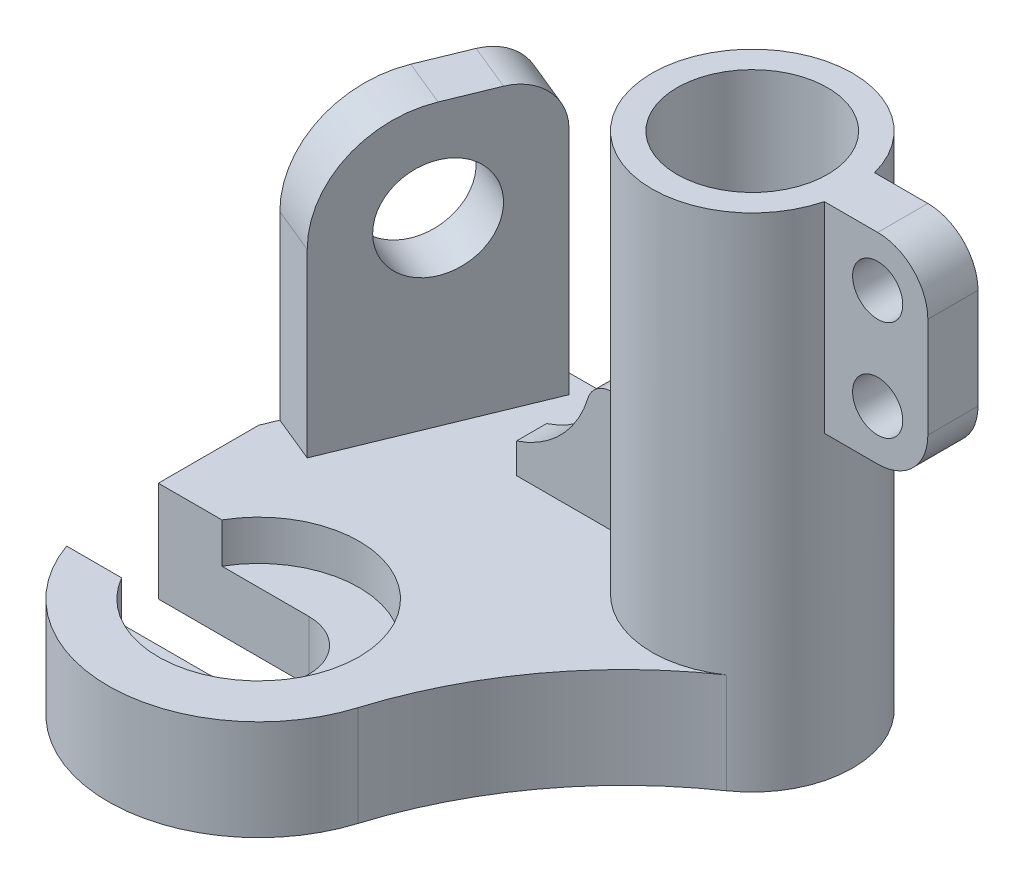
ISO-10303-21;
HEADER;
FILE_DESCRIPTION(('STEP AP214'),'2;1');
FILE_NAME('part.step','',(''),(''),'','','');
FILE_SCHEMA(('AUTOMOTIVE_DESIGN { 1 0 10303 214 1 1 1 1 }'));
ENDSEC;
DATA;
#1=APPLICATION_CONTEXT('core data for automotive mechanical design processes');
#2=APPLICATION_PROTOCOL_DEFINITION('international standard','automotive_design',2000,#1);
#3=PRODUCT_CONTEXT('',#1,'mechanical');
#4=PRODUCT('Part','Part','',(#3));
#5=PRODUCT_RELATED_PRODUCT_CATEGORY('part','',(#4));
#6=PRODUCT_DEFINITION_FORMATION('','',#4);
#7=PRODUCT_DEFINITION_CONTEXT('part definition',#1,'design');
#8=PRODUCT_DEFINITION('design','',#6,#7);
#9=PRODUCT_DEFINITION_SHAPE('','',#8);
#10=(LENGTH_UNIT() NAMED_UNIT(*) SI_UNIT(.MILLI.,.METRE.));
#11=(NAMED_UNIT(*) PLANE_ANGLE_UNIT() SI_UNIT($,.RADIAN.));
#12=(NAMED_UNIT(*) SI_UNIT($,.STERADIAN.) SOLID_ANGLE_UNIT());
#13=UNCERTAINTY_MEASURE_WITH_UNIT(LENGTH_MEASURE(1.E-05),#10,'distance_accuracy_value','');
#14=(GEOMETRIC_REPRESENTATION_CONTEXT(3) GLOBAL_UNCERTAINTY_ASSIGNED_CONTEXT((#13)) GLOBAL_UNIT_ASSIGNED_CONTEXT((#10,
#11,#12)) REPRESENTATION_CONTEXT('',''));
#15=CARTESIAN_POINT('',(0.,0.,0.));
#16=DIRECTION('',(0.,0.,1.));
#17=DIRECTION('',(1.,0.,0.));
#18=AXIS2_PLACEMENT_3D('',#15,#16,#17);
#19=CARTESIAN_POINT('',(-48.41,0.,50.));
#20=DIRECTION('',(0.,1.,0.));
#21=DIRECTION('',(0.,0.,1.));
#22=AXIS2_PLACEMENT_3D('',#19,#20,#21);
#23=CYLINDRICAL_SURFACE('',#22,10.);
#24=CARTESIAN_POINT('',(-48.41,12.,50.));
#25=DIRECTION('',(0.,1.,0.));
#26=DIRECTION('',(0.,0.,1.));
#27=AXIS2_PLACEMENT_3D('',#24,#25,#26);
#28=CIRCLE('',#27,10.);
#29=CARTESIAN_POINT('',(-48.41,12.,40.));
#30=VERTEX_POINT('',#29);
#31=CARTESIAN_POINT('',(-48.41,12.,60.));
#32=VERTEX_POINT('',#31);
#33=EDGE_CURVE('E314',#30,#32,#28,.F.);
#34=ORIENTED_EDGE('',*,*,#33,.F.);
#35=DIRECTION('',(0.,1.,0.));
#36=VECTOR('',#35,1.);
#37=CARTESIAN_POINT('',(-48.41,0.,40.));
#38=LINE('',#37,#36);
#39=CARTESIAN_POINT('',(-48.41,0.,40.));
#40=VERTEX_POINT('',#39);
#41=EDGE_CURVE('E335',#40,#30,#38,.T.);
#42=ORIENTED_EDGE('',*,*,#41,.F.);
#43=CARTESIAN_POINT('',(-48.41,0.,50.));
#44=DIRECTION('',(0.,1.,0.));
#45=DIRECTION('',(0.,0.,1.));
#46=AXIS2_PLACEMENT_3D('',#43,#44,#45);
#47=CIRCLE('',#46,10.);
#48=CARTESIAN_POINT('',(-48.41,0.,60.));
#49=VERTEX_POINT('',#48);
#50=EDGE_CURVE('E323',#49,#40,#47,.T.);
#51=ORIENTED_EDGE('',*,*,#50,.F.);
#52=DIRECTION('',(0.,1.,0.));
#53=VECTOR('',#52,1.);
#54=CARTESIAN_POINT('',(-48.41,0.,60.));
#55=LINE('',#54,#53);
#56=EDGE_CURVE('E331',#49,#32,#55,.T.);
#57=ORIENTED_EDGE('',*,*,#56,.T.);
#58=EDGE_LOOP('',(#34,#42,#51,#57));
#59=FACE_BOUND('',#58,.T.);
#60=ADVANCED_FACE('F39',(#59),#23,.F.);
#61=CARTESIAN_POINT('',(0.,100.,0.));
#62=DIRECTION('',(0.,-1.,0.));
#63=DIRECTION('',(0.,0.,-1.));
#64=AXIS2_PLACEMENT_3D('',#61,#62,#63);
#65=CYLINDRICAL_SURFACE('',#64,20.);
#66=CARTESIAN_POINT('',(0.,100.,0.));
#67=DIRECTION('',(0.,1.,0.));
#68=DIRECTION('',(0.,0.,1.));
#69=AXIS2_PLACEMENT_3D('',#66,#67,#68);
#70=CIRCLE('',#69,20.);
#71=CARTESIAN_POINT('',(19.3649167310371,100.,-5.));
#72=VERTEX_POINT('',#71);
#73=CARTESIAN_POINT('',(19.3649167310371,100.,5.));
#74=VERTEX_POINT('',#73);
#75=EDGE_CURVE('E450',#72,#74,#70,.T.);
#76=ORIENTED_EDGE('',*,*,#75,.F.);
#77=DIRECTION('',(0.,-1.,0.));
#78=VECTOR('',#77,1.);
#79=CARTESIAN_POINT('',(19.3649167310371,100.,-5.));
#80=LINE('',#79,#78);
#81=CARTESIAN_POINT('',(19.3649167310371,60.,-5.));
#82=VERTEX_POINT('',#81);
#83=EDGE_CURVE('E306',#72,#82,#80,.T.);
#84=ORIENTED_EDGE('',*,*,#83,.T.);
#85=CARTESIAN_POINT('',(0.,60.,0.));
#86=DIRECTION('',(0.,1.,0.));
#87=DIRECTION('',(0.,0.,1.));
#88=AXIS2_PLACEMENT_3D('',#85,#86,#87);
#89=CIRCLE('',#88,20.);
#90=CARTESIAN_POINT('',(19.3649167310371,60.,5.));
#91=VERTEX_POINT('',#90);
#92=EDGE_CURVE('E459',#91,#82,#89,.T.);
#93=ORIENTED_EDGE('',*,*,#92,.F.);
#94=DIRECTION('',(0.,-1.,0.));
#95=VECTOR('',#94,1.);
#96=CARTESIAN_POINT('',(19.3649167310371,100.,5.));
#97=LINE('',#96,#95);
#98=EDGE_CURVE('E303',#91,#74,#97,.F.);
#99=ORIENTED_EDGE('',*,*,#98,.T.);
#100=EDGE_LOOP('',(#76,#84,#93,#99));
#101=FACE_BOUND('',#100,.T.);
#102=CARTESIAN_POINT('',(0.,44.,0.));
#103=DIRECTION('',(0.,-1.,0.));
#104=DIRECTION('',(0.,0.,-1.));
#105=AXIS2_PLACEMENT_3D('',#102,#103,#104);
#106=CIRCLE('',#105,20.);
#107=CARTESIAN_POINT('',(-19.7737199332852,44.,3.));
#108=VERTEX_POINT('',#107);
#109=CARTESIAN_POINT('',(-19.7737199332852,44.,-3.));
#110=VERTEX_POINT('',#109);
#111=EDGE_CURVE('E11',#108,#110,#106,.T.);
#112=ORIENTED_EDGE('',*,*,#111,.F.);
#113=DIRECTION('',(0.,-1.,0.));
#114=VECTOR('',#113,1.);
#115=CARTESIAN_POINT('',(-19.7737199332852,100.,3.));
#116=LINE('',#115,#114);
#117=CARTESIAN_POINT('',(-19.7737199332852,20.,3.));
#118=VERTEX_POINT('',#117);
#119=EDGE_CURVE('E236',#108,#118,#116,.T.);
#120=ORIENTED_EDGE('',*,*,#119,.T.);
#121=CARTESIAN_POINT('',(0.,20.,0.));
#122=DIRECTION('',(0.,-1.,0.));
#123=DIRECTION('',(0.,0.,1.));
#124=AXIS2_PLACEMENT_3D('',#121,#122,#123);
#125=CIRCLE('',#124,20.);
#126=CARTESIAN_POINT('',(11.3447753734864,20.,16.4710677166095));
#127=VERTEX_POINT('',#126);
#128=EDGE_CURVE('E404',#127,#118,#125,.T.);
#129=ORIENTED_EDGE('',*,*,#128,.F.);
#130=DIRECTION('',(0.,-1.,0.));
#131=VECTOR('',#130,1.);
#132=CARTESIAN_POINT('',(11.3447753734864,20.,16.4710677166095));
#133=LINE('',#132,#131);
#134=CARTESIAN_POINT('',(11.3447753734864,0.,16.4710677166095));
#135=VERTEX_POINT('',#134);
#136=EDGE_CURVE('E419',#127,#135,#133,.T.);
#137=ORIENTED_EDGE('',*,*,#136,.T.);
#138=CARTESIAN_POINT('',(0.,0.,0.));
#139=DIRECTION('',(0.,1.,0.));
#140=DIRECTION('',(0.,0.,1.));
#141=AXIS2_PLACEMENT_3D('',#138,#139,#140);
#142=CIRCLE('',#141,20.);
#143=CARTESIAN_POINT('',(0.,0.,-20.));
#144=VERTEX_POINT('',#143);
#145=EDGE_CURVE('E447',#135,#144,#142,.T.);
#146=ORIENTED_EDGE('',*,*,#145,.T.);
#147=DIRECTION('',(0.,-1.,0.));
#148=VECTOR('',#147,1.);
#149=CARTESIAN_POINT('',(0.,20.,-20.));
#150=LINE('',#149,#148);
#151=CARTESIAN_POINT('',(0.,20.,-20.));
#152=VERTEX_POINT('',#151);
#153=EDGE_CURVE('E444',#152,#144,#150,.T.);
#154=ORIENTED_EDGE('',*,*,#153,.F.);
#155=CARTESIAN_POINT('',(-19.7737199332852,20.,-3.));
#156=VERTEX_POINT('',#155);
#157=EDGE_CURVE('E408',#156,#152,#125,.T.);
#158=ORIENTED_EDGE('',*,*,#157,.F.);
#159=DIRECTION('',(0.,-1.,0.));
#160=VECTOR('',#159,1.);
#161=CARTESIAN_POINT('',(-19.7737199332852,100.,-3.));
#162=LINE('',#161,#160);
#163=EDGE_CURVE('E53',#110,#156,#162,.T.);
#164=ORIENTED_EDGE('',*,*,#163,.F.);
#165=EDGE_LOOP('',(#112,#120,#129,#137,#146,#154,#158,#164));
#166=FACE_BOUND('',#165,.T.);
#167=ADVANCED_FACE('F489',(#101,#166),#65,.T.);
#168=CARTESIAN_POINT('',(0.,100.,0.));
#169=DIRECTION('',(0.,1.,0.));
#170=DIRECTION('',(0.,0.,1.));
#171=AXIS2_PLACEMENT_3D('',#168,#169,#170);
#172=PLANE('',#171);
#173=DIRECTION('',(1.,0.,0.));
#174=VECTOR('',#173,1.);
#175=CARTESIAN_POINT('',(18.5219863965461,100.,5.));
#176=LINE('',#175,#174);
#177=CARTESIAN_POINT('',(30.,100.,5.));
#178=VERTEX_POINT('',#177);
#179=EDGE_CURVE('E292',#74,#178,#176,.T.);
#180=ORIENTED_EDGE('',*,*,#179,.T.);
#181=DIRECTION('',(0.,0.,-1.));
#182=VECTOR('',#181,1.);
#183=CARTESIAN_POINT('',(30.,100.,0.));
#184=LINE('',#183,#182);
#185=CARTESIAN_POINT('',(30.,100.,-5.));
#186=VERTEX_POINT('',#185);
#187=EDGE_CURVE('E50',#178,#186,#184,.T.);
#188=ORIENTED_EDGE('',*,*,#187,.T.);
#189=DIRECTION('',(-1.,0.,0.));
#190=VECTOR('',#189,1.);
#191=CARTESIAN_POINT('',(18.5219863965461,100.,-5.));
#192=LINE('',#191,#190);
#193=EDGE_CURVE('E297',#186,#72,#192,.T.);
#194=ORIENTED_EDGE('',*,*,#193,.T.);
#195=ORIENTED_EDGE('',*,*,#75,.T.);
#196=EDGE_LOOP('',(#180,#188,#194,#195));
#197=FACE_BOUND('',#196,.T.);
#198=CARTESIAN_POINT('',(0.,100.,0.));
#199=DIRECTION('',(0.,1.,0.));
#200=DIRECTION('',(0.,0.,1.));
#201=AXIS2_PLACEMENT_3D('',#198,#199,#200);
#202=CIRCLE('',#201,15.);
#203=CARTESIAN_POINT('',(0.,100.,15.));
#204=VERTEX_POINT('',#203);
#205=EDGE_CURVE('E390',#204,#204,#202,.T.);
#206=ORIENTED_EDGE('',*,*,#205,.F.);
#207=EDGE_LOOP('',(#206));
#208=FACE_BOUND('',#207,.T.);
#209=ADVANCED_FACE('F479',(#197,#208),#172,.T.);
#210=CARTESIAN_POINT('',(0.,0.,0.));
#211=DIRECTION('',(0.,1.,0.));
#212=DIRECTION('',(0.,0.,1.));
#213=AXIS2_PLACEMENT_3D('',#210,#211,#212);
#214=PLANE('',#213);
#215=CARTESIAN_POINT('',(-48.41,0.,50.));
#216=DIRECTION('',(0.,1.,0.));
#217=DIRECTION('',(0.,0.,1.));
#218=AXIS2_PLACEMENT_3D('',#215,#216,#217);
#219=CIRCLE('',#218,30.);
#220=CARTESIAN_POINT('',(-76.6942712474619,0.,60.));
#221=VERTEX_POINT('',#220);
#222=CARTESIAN_POINT('',(-19.7371244907003,0.,58.8241832499221));
#223=VERTEX_POINT('',#222);
#224=EDGE_CURVE('E430',#221,#223,#219,.T.);
#225=ORIENTED_EDGE('',*,*,#224,.F.);
#226=DIRECTION('',(1.,0.,0.));
#227=VECTOR('',#226,1.);
#228=CARTESIAN_POINT('',(-48.41,0.,60.));
#229=LINE('',#228,#227);
#230=EDGE_CURVE('E328',#221,#49,#229,.T.);
#231=ORIENTED_EDGE('',*,*,#230,.T.);
#232=ORIENTED_EDGE('',*,*,#50,.T.);
#233=DIRECTION('',(-1.,0.,0.));
#234=VECTOR('',#233,1.);
#235=CARTESIAN_POINT('',(-48.41,0.,40.));
#236=LINE('',#235,#234);
#237=CARTESIAN_POINT('',(-78.41,0.,40.));
#238=VERTEX_POINT('',#237);
#239=EDGE_CURVE('E326',#40,#238,#236,.T.);
#240=ORIENTED_EDGE('',*,*,#239,.T.);
#241=DIRECTION('',(0.,0.,1.));
#242=VECTOR('',#241,1.);
#243=CARTESIAN_POINT('',(-78.41,0.,20.));
#244=LINE('',#243,#242);
#245=CARTESIAN_POINT('',(-78.41,0.,20.));
#246=VERTEX_POINT('',#245);
#247=EDGE_CURVE('E424',#246,#238,#244,.T.);
#248=ORIENTED_EDGE('',*,*,#247,.F.);
#249=DIRECTION('',(-0.379551280046691,0.,0.92517070090601));
#250=VECTOR('',#249,1.);
#251=CARTESIAN_POINT('',(-62.,0.,-20.));
#252=LINE('',#251,#250);
#253=CARTESIAN_POINT('',(-62.,0.,-20.));
#254=VERTEX_POINT('',#253);
#255=EDGE_CURVE('E425',#254,#246,#252,.T.);
#256=ORIENTED_EDGE('',*,*,#255,.F.);
#257=DIRECTION('',(-1.,0.,0.));
#258=VECTOR('',#257,1.);
#259=CARTESIAN_POINT('',(0.,0.,-20.));
#260=LINE('',#259,#258);
#261=EDGE_CURVE('E401',#144,#254,#260,.T.);
#262=ORIENTED_EDGE('',*,*,#261,.F.);
#263=ORIENTED_EDGE('',*,*,#145,.F.);
#264=CARTESIAN_POINT('',(56.723876867432,0.,82.3553385830477));
#265=DIRECTION('',(0.,-1.,0.));
#266=DIRECTION('',(0.,0.,-1.));
#267=AXIS2_PLACEMENT_3D('',#264,#265,#266);
#268=CIRCLE('',#267,80.);
#269=EDGE_CURVE('E427',#223,#135,#268,.T.);
#270=ORIENTED_EDGE('',*,*,#269,.F.);
#271=EDGE_LOOP('',(#225,#231,#232,#240,#248,#256,#262,#263,#270));
#272=FACE_BOUND('',#271,.T.);
#273=ADVANCED_FACE('F586',(#272),#214,.F.);
#274=CARTESIAN_POINT('',(0.,20.,-20.));
#275=DIRECTION('',(0.,0.,1.));
#276=DIRECTION('',(1.,0.,0.));
#277=AXIS2_PLACEMENT_3D('',#274,#275,#276);
#278=PLANE('',#277);
#279=ORIENTED_EDGE('',*,*,#261,.T.);
#280=DIRECTION('',(0.,-1.,0.));
#281=VECTOR('',#280,1.);
#282=CARTESIAN_POINT('',(-62.,20.,-20.));
#283=LINE('',#282,#281);
#284=CARTESIAN_POINT('',(-62.,20.,-20.));
#285=VERTEX_POINT('',#284);
#286=EDGE_CURVE('E439',#285,#254,#283,.T.);
#287=ORIENTED_EDGE('',*,*,#286,.F.);
#288=DIRECTION('',(-1.,0.,0.));
#289=VECTOR('',#288,1.);
#290=CARTESIAN_POINT('',(0.,20.,-20.));
#291=LINE('',#290,#289);
#292=EDGE_CURVE('E410',#152,#285,#291,.T.);
#293=ORIENTED_EDGE('',*,*,#292,.F.);
#294=ORIENTED_EDGE('',*,*,#153,.T.);
#295=EDGE_LOOP('',(#279,#287,#293,#294));
#296=FACE_BOUND('',#295,.T.);
#297=ADVANCED_FACE('F585',(#296),#278,.F.);
#298=CARTESIAN_POINT('',(-62.,20.,-20.));
#299=DIRECTION('',(0.925170700906011,0.,0.379551280046691));
#300=DIRECTION('',(0.379551280046691,0.,-0.925170700906011));
#301=AXIS2_PLACEMENT_3D('',#298,#299,#300);
#302=PLANE('',#301);
#303=ORIENTED_EDGE('',*,*,#255,.T.);
#304=DIRECTION('',(0.,-1.,0.));
#305=VECTOR('',#304,1.);
#306=CARTESIAN_POINT('',(-78.41,20.,20.));
#307=LINE('',#306,#305);
#308=CARTESIAN_POINT('',(-78.41,20.,20.));
#309=VERTEX_POINT('',#308);
#310=EDGE_CURVE('E440',#309,#246,#307,.T.);
#311=ORIENTED_EDGE('',*,*,#310,.F.);
#312=DIRECTION('',(-0.379551280046691,0.,0.92517070090601));
#313=VECTOR('',#312,1.);
#314=CARTESIAN_POINT('',(-62.,20.,-20.));
#315=LINE('',#314,#313);
#316=CARTESIAN_POINT('',(-77.1820512018676,20.,17.0068280362404));
#317=VERTEX_POINT('',#316);
#318=EDGE_CURVE('E406',#317,#309,#315,.T.);
#319=ORIENTED_EDGE('',*,*,#318,.F.);
#320=DIRECTION('',(0.,1.,0.));
#321=VECTOR('',#320,1.);
#322=CARTESIAN_POINT('',(-77.1820512018676,56.,17.0068280362404));
#323=LINE('',#322,#321);
#324=CARTESIAN_POINT('',(-77.1820512018676,56.,17.0068280362404));
#325=VERTEX_POINT('',#324);
#326=EDGE_CURVE('E349',#317,#325,#323,.T.);
#327=ORIENTED_EDGE('',*,*,#326,.T.);
#328=CARTESIAN_POINT('',(-69.5910256009338,56.,-1.49658598187978));
#329=DIRECTION('',(-0.925170700906011,0.,-0.379551280046691));
#330=DIRECTION('',(0.379551280046691,0.,-0.925170700906011));
#331=AXIS2_PLACEMENT_3D('',#328,#329,#330);
#332=CIRCLE('',#331,20.);
#333=CARTESIAN_POINT('',(-69.5910256009338,76.,-1.49658598187978));
#334=VERTEX_POINT('',#333);
#335=EDGE_CURVE('E373',#325,#334,#332,.T.);
#336=ORIENTED_EDGE('',*,*,#335,.T.);
#337=DIRECTION('',(0.379551280046691,0.,-0.92517070090601));
#338=VECTOR('',#337,1.);
#339=CARTESIAN_POINT('',(-65.7955128004669,76.,-10.7482929909398));
#340=LINE('',#339,#338);
#341=CARTESIAN_POINT('',(-65.7955128004669,76.,-10.7482929909398));
#342=VERTEX_POINT('',#341);
#343=EDGE_CURVE('E376',#334,#342,#340,.T.);
#344=ORIENTED_EDGE('',*,*,#343,.T.);
#345=CARTESIAN_POINT('',(-65.7955128004669,66.,-10.7482929909399));
#346=DIRECTION('',(-0.925170700906011,0.,-0.379551280046691));
#347=DIRECTION('',(0.379551280046691,0.,-0.925170700906011));
#348=AXIS2_PLACEMENT_3D('',#345,#346,#347);
#349=CIRCLE('',#348,10.);
#350=CARTESIAN_POINT('',(-62.,65.9999999999999,-20.));
#351=VERTEX_POINT('',#350);
#352=EDGE_CURVE('E377',#342,#351,#349,.T.);
#353=ORIENTED_EDGE('',*,*,#352,.T.);
#354=DIRECTION('',(0.,-1.,0.));
#355=VECTOR('',#354,1.);
#356=CARTESIAN_POINT('',(-62.,20.,-20.));
#357=LINE('',#356,#355);
#358=EDGE_CURVE('E351',#351,#285,#357,.T.);
#359=ORIENTED_EDGE('',*,*,#358,.T.);
#360=ORIENTED_EDGE('',*,*,#286,.T.);
#361=EDGE_LOOP('',(#303,#311,#319,#327,#336,#344,#353,#359,#360));
#362=FACE_BOUND('',#361,.T.);
#363=CARTESIAN_POINT('',(-69.5910256009338,56.,-1.49658598187978));
#364=DIRECTION('',(-0.925170700906011,0.,-0.379551280046691));
#365=DIRECTION('',(-0.379551280046691,0.,0.925170700906011));
#366=AXIS2_PLACEMENT_3D('',#363,#364,#365);
#367=CIRCLE('',#366,10.);
#368=CARTESIAN_POINT('',(-73.3865384014007,56.,7.75512102718032));
#369=VERTEX_POINT('',#368);
#370=EDGE_CURVE('E342',#369,#369,#367,.T.);
#371=ORIENTED_EDGE('',*,*,#370,.F.);
#372=EDGE_LOOP('',(#371));
#373=FACE_BOUND('',#372,.T.);
#374=ADVANCED_FACE('F577',(#362,#373),#302,.F.);
#375=CARTESIAN_POINT('',(-78.41,20.,20.));
#376=DIRECTION('',(1.,0.,0.));
#377=DIRECTION('',(0.,0.,-1.));
#378=AXIS2_PLACEMENT_3D('',#375,#376,#377);
#379=PLANE('',#378);
#380=ORIENTED_EDGE('',*,*,#247,.T.);
#381=DIRECTION('',(0.,1.,0.));
#382=VECTOR('',#381,1.);
#383=CARTESIAN_POINT('',(-78.41,0.,40.));
#384=LINE('',#383,#382);
#385=CARTESIAN_POINT('',(-78.41,20.,40.));
#386=VERTEX_POINT('',#385);
#387=EDGE_CURVE('E338',#238,#386,#384,.T.);
#388=ORIENTED_EDGE('',*,*,#387,.T.);
#389=DIRECTION('',(0.,0.,1.));
#390=VECTOR('',#389,1.);
#391=CARTESIAN_POINT('',(-78.41,20.,20.));
#392=LINE('',#391,#390);
#393=EDGE_CURVE('E411',#309,#386,#392,.T.);
#394=ORIENTED_EDGE('',*,*,#393,.F.);
#395=ORIENTED_EDGE('',*,*,#310,.T.);
#396=EDGE_LOOP('',(#380,#388,#394,#395));
#397=FACE_BOUND('',#396,.T.);
#398=ADVANCED_FACE('F579',(#397),#379,.F.);
#399=CARTESIAN_POINT('',(-48.41,20.,50.));
#400=DIRECTION('',(0.,-1.,0.));
#401=DIRECTION('',(0.,0.,-1.));
#402=AXIS2_PLACEMENT_3D('',#399,#400,#401);
#403=CYLINDRICAL_SURFACE('',#402,30.);
#404=CARTESIAN_POINT('',(-48.41,20.,50.));
#405=DIRECTION('',(0.,1.,0.));
#406=DIRECTION('',(0.,0.,1.));
#407=AXIS2_PLACEMENT_3D('',#404,#405,#406);
#408=CIRCLE('',#407,30.);
#409=CARTESIAN_POINT('',(-76.6942712474619,20.,60.));
#410=VERTEX_POINT('',#409);
#411=CARTESIAN_POINT('',(-19.7371244907003,20.,58.8241832499221));
#412=VERTEX_POINT('',#411);
#413=EDGE_CURVE('E412',#410,#412,#408,.T.);
#414=ORIENTED_EDGE('',*,*,#413,.F.);
#415=DIRECTION('',(0.,-1.,0.));
#416=VECTOR('',#415,1.);
#417=CARTESIAN_POINT('',(-76.6942712474619,20.,60.));
#418=LINE('',#417,#416);
#419=EDGE_CURVE('E340',#410,#221,#418,.T.);
#420=ORIENTED_EDGE('',*,*,#419,.T.);
#421=ORIENTED_EDGE('',*,*,#224,.T.);
#422=DIRECTION('',(0.,-1.,0.));
#423=VECTOR('',#422,1.);
#424=CARTESIAN_POINT('',(-19.7371244907003,20.,58.8241832499221));
#425=LINE('',#424,#423);
#426=EDGE_CURVE('E432',#412,#223,#425,.T.);
#427=ORIENTED_EDGE('',*,*,#426,.F.);
#428=EDGE_LOOP('',(#414,#420,#421,#427));
#429=FACE_BOUND('',#428,.T.);
#430=ADVANCED_FACE('F573',(#429),#403,.T.);
#431=CARTESIAN_POINT('',(56.723876867432,20.,82.3553385830477));
#432=DIRECTION('',(0.,-1.,0.));
#433=DIRECTION('',(0.,0.,-1.));
#434=AXIS2_PLACEMENT_3D('',#431,#432,#433);
#435=CYLINDRICAL_SURFACE('',#434,80.);
#436=ORIENTED_EDGE('',*,*,#269,.T.);
#437=ORIENTED_EDGE('',*,*,#136,.F.);
#438=CARTESIAN_POINT('',(56.723876867432,20.,82.3553385830477));
#439=DIRECTION('',(0.,-1.,0.));
#440=DIRECTION('',(0.,0.,-1.));
#441=AXIS2_PLACEMENT_3D('',#438,#439,#440);
#442=CIRCLE('',#441,80.);
#443=EDGE_CURVE('E417',#412,#127,#442,.T.);
#444=ORIENTED_EDGE('',*,*,#443,.F.);
#445=ORIENTED_EDGE('',*,*,#426,.T.);
#446=EDGE_LOOP('',(#436,#437,#444,#445));
#447=FACE_BOUND('',#446,.T.);
#448=ADVANCED_FACE('F569',(#447),#435,.F.);
#449=CARTESIAN_POINT('',(0.,20.,0.));
#450=DIRECTION('',(0.,1.,0.));
#451=DIRECTION('',(0.,0.,1.));
#452=AXIS2_PLACEMENT_3D('',#449,#450,#451);
#453=PLANE('',#452);
#454=DIRECTION('',(1.,0.,0.));
#455=VECTOR('',#454,1.);
#456=CARTESIAN_POINT('',(-44.,20.,3.));
#457=LINE('',#456,#455);
#458=CARTESIAN_POINT('',(-44.,20.,3.));
#459=VERTEX_POINT('',#458);
#460=EDGE_CURVE('E242',#459,#118,#457,.T.);
#461=ORIENTED_EDGE('',*,*,#460,.F.);
#462=DIRECTION('',(0.,0.,-1.));
#463=VECTOR('',#462,1.);
#464=CARTESIAN_POINT('',(-44.,20.,3.));
#465=LINE('',#464,#463);
#466=CARTESIAN_POINT('',(-44.,20.,-3.));
#467=VERTEX_POINT('',#466);
#468=EDGE_CURVE('E261',#459,#467,#465,.T.);
#469=ORIENTED_EDGE('',*,*,#468,.T.);
#470=DIRECTION('',(1.,0.,0.));
#471=VECTOR('',#470,1.);
#472=CARTESIAN_POINT('',(-44.,20.,-3.));
#473=LINE('',#472,#471);
#474=EDGE_CURVE('E265',#467,#156,#473,.T.);
#475=ORIENTED_EDGE('',*,*,#474,.T.);
#476=ORIENTED_EDGE('',*,*,#157,.T.);
#477=ORIENTED_EDGE('',*,*,#292,.T.);
#478=DIRECTION('',(-0.925170700906011,0.,-0.379551280046691));
#479=VECTOR('',#478,1.);
#480=CARTESIAN_POINT('',(-52.7482929909399,20.,-16.2044871995331));
#481=LINE('',#480,#479);
#482=CARTESIAN_POINT('',(-52.7482929909399,20.,-16.2044871995331));
#483=VERTEX_POINT('',#482);
#484=EDGE_CURVE('E383',#483,#285,#481,.T.);
#485=ORIENTED_EDGE('',*,*,#484,.F.);
#486=DIRECTION('',(-0.379551280046691,0.,0.92517070090601));
#487=VECTOR('',#486,1.);
#488=CARTESIAN_POINT('',(-67.9303441928075,20.,20.8023408367073));
#489=LINE('',#488,#487);
#490=CARTESIAN_POINT('',(-67.9303441928075,20.,20.8023408367073));
#491=VERTEX_POINT('',#490);
#492=EDGE_CURVE('E355',#483,#491,#489,.T.);
#493=ORIENTED_EDGE('',*,*,#492,.T.);
#494=DIRECTION('',(-0.925170700906011,0.,-0.379551280046691));
#495=VECTOR('',#494,1.);
#496=CARTESIAN_POINT('',(-67.9303441928075,20.,20.8023408367073));
#497=LINE('',#496,#495);
#498=EDGE_CURVE('E367',#491,#317,#497,.T.);
#499=ORIENTED_EDGE('',*,*,#498,.T.);
#500=ORIENTED_EDGE('',*,*,#318,.T.);
#501=ORIENTED_EDGE('',*,*,#393,.T.);
#502=DIRECTION('',(-1.,0.,0.));
#503=VECTOR('',#502,1.);
#504=CARTESIAN_POINT('',(-48.41,20.,40.));
#505=LINE('',#504,#503);
#506=CARTESIAN_POINT('',(-65.7305080756888,20.,40.));
#507=VERTEX_POINT('',#506);
#508=EDGE_CURVE('E325',#507,#386,#505,.T.);
#509=ORIENTED_EDGE('',*,*,#508,.F.);
#510=CARTESIAN_POINT('',(-48.41,20.,50.));
#511=DIRECTION('',(0.,1.,0.));
#512=DIRECTION('',(0.,0.,1.));
#513=AXIS2_PLACEMENT_3D('',#510,#511,#512);
#514=CIRCLE('',#513,20.);
#515=CARTESIAN_POINT('',(-65.7305080756888,20.,60.));
#516=VERTEX_POINT('',#515);
#517=EDGE_CURVE('E313',#516,#507,#514,.T.);
#518=ORIENTED_EDGE('',*,*,#517,.F.);
#519=DIRECTION('',(1.,0.,0.));
#520=VECTOR('',#519,1.);
#521=CARTESIAN_POINT('',(0.,20.,60.));
#522=LINE('',#521,#520);
#523=EDGE_CURVE('E446',#410,#516,#522,.T.);
#524=ORIENTED_EDGE('',*,*,#523,.F.);
#525=ORIENTED_EDGE('',*,*,#413,.T.);
#526=ORIENTED_EDGE('',*,*,#443,.T.);
#527=ORIENTED_EDGE('',*,*,#128,.T.);
#528=EDGE_LOOP('',(#461,#469,#475,#476,#477,#485,#493,#499,#500,#501,#509,#518,#524,#525,#526,#527));
#529=FACE_BOUND('',#528,.T.);
#530=ADVANCED_FACE('F562',(#529),#453,.T.);
#531=CARTESIAN_POINT('',(0.,58.,0.));
#532=DIRECTION('',(0.,1.,0.));
#533=DIRECTION('',(0.,0.,1.));
#534=AXIS2_PLACEMENT_3D('',#531,#532,#533);
#535=CONICAL_SURFACE('',#534,15.,1.02974425867665);
#536=CARTESIAN_POINT('',(0.,48.9870907145866,0.));
#537=VERTEX_POINT('',#536);
#538=VERTEX_LOOP('',#537);
#539=FACE_BOUND('',#538,.T.);
#540=CARTESIAN_POINT('',(0.,58.,0.));
#541=DIRECTION('',(0.,1.,0.));
#542=DIRECTION('',(0.,0.,1.));
#543=AXIS2_PLACEMENT_3D('',#540,#541,#542);
#544=CIRCLE('',#543,15.);
#545=CARTESIAN_POINT('',(0.,58.,15.));
#546=VERTEX_POINT('',#545);
#547=EDGE_CURVE('E397',#546,#546,#544,.T.);
#548=ORIENTED_EDGE('',*,*,#547,.T.);
#549=EDGE_LOOP('',(#548));
#550=FACE_BOUND('',#549,.T.);
#551=ADVANCED_FACE('F564',(#539,#550),#535,.F.);
#552=CARTESIAN_POINT('',(0.,100.,0.));
#553=DIRECTION('',(0.,1.,0.));
#554=DIRECTION('',(0.,0.,1.));
#555=AXIS2_PLACEMENT_3D('',#552,#553,#554);
#556=CYLINDRICAL_SURFACE('',#555,15.);
#557=ORIENTED_EDGE('',*,*,#547,.F.);
#558=EDGE_LOOP('',(#557));
#559=FACE_BOUND('',#558,.T.);
#560=ORIENTED_EDGE('',*,*,#205,.T.);
#561=EDGE_LOOP('',(#560));
#562=FACE_BOUND('',#561,.T.);
#563=ADVANCED_FACE('F543',(#559,#562),#556,.F.);
#564=CARTESIAN_POINT('',(-52.7482929909399,20.,-16.2044871995331));
#565=DIRECTION('',(0.379551280046691,0.,-0.925170700906011));
#566=DIRECTION('',(-0.925170700906011,0.,-0.379551280046691));
#567=AXIS2_PLACEMENT_3D('',#564,#565,#566);
#568=PLANE('',#567);
#569=ORIENTED_EDGE('',*,*,#358,.F.);
#570=DIRECTION('',(-0.925170700906011,0.,-0.379551280046691));
#571=VECTOR('',#570,1.);
#572=CARTESIAN_POINT('',(-52.7482929909399,65.9999999999999,-16.2044871995331));
#573=LINE('',#572,#571);
#574=CARTESIAN_POINT('',(-52.7482929909399,65.9999999999999,-16.2044871995331));
#575=VERTEX_POINT('',#574);
#576=EDGE_CURVE('E389',#575,#351,#573,.T.);
#577=ORIENTED_EDGE('',*,*,#576,.F.);
#578=DIRECTION('',(0.,-1.,0.));
#579=VECTOR('',#578,1.);
#580=CARTESIAN_POINT('',(-52.7482929909399,20.,-16.2044871995331));
#581=LINE('',#580,#579);
#582=EDGE_CURVE('E370',#575,#483,#581,.T.);
#583=ORIENTED_EDGE('',*,*,#582,.T.);
#584=ORIENTED_EDGE('',*,*,#484,.T.);
#585=EDGE_LOOP('',(#569,#577,#583,#584));
#586=FACE_BOUND('',#585,.T.);
#587=ADVANCED_FACE('F537',(#586),#568,.T.);
#588=CARTESIAN_POINT('',(-56.5438057914068,66.,-6.95278019047298));
#589=DIRECTION('',(-0.925170700906011,0.,-0.379551280046691));
#590=DIRECTION('',(-0.379551280046691,0.,0.925170700906011));
#591=AXIS2_PLACEMENT_3D('',#588,#589,#590);
#592=CYLINDRICAL_SURFACE('',#591,10.);
#593=ORIENTED_EDGE('',*,*,#352,.F.);
#594=DIRECTION('',(-0.925170700906011,0.,-0.379551280046691));
#595=VECTOR('',#594,1.);
#596=CARTESIAN_POINT('',(-56.5438057914068,76.,-6.95278019047292));
#597=LINE('',#596,#595);
#598=CARTESIAN_POINT('',(-56.5438057914068,76.,-6.95278019047292));
#599=VERTEX_POINT('',#598);
#600=EDGE_CURVE('E388',#599,#342,#597,.T.);
#601=ORIENTED_EDGE('',*,*,#600,.F.);
#602=CARTESIAN_POINT('',(-56.5438057914068,66.,-6.95278019047298));
#603=DIRECTION('',(-0.925170700906011,0.,-0.379551280046691));
#604=DIRECTION('',(0.379551280046691,0.,-0.925170700906011));
#605=AXIS2_PLACEMENT_3D('',#602,#603,#604);
#606=CIRCLE('',#605,10.);
#607=EDGE_CURVE('E365',#599,#575,#606,.T.);
#608=ORIENTED_EDGE('',*,*,#607,.T.);
#609=ORIENTED_EDGE('',*,*,#576,.T.);
#610=EDGE_LOOP('',(#593,#601,#608,#609));
#611=FACE_BOUND('',#610,.T.);
#612=ADVANCED_FACE('F545',(#611),#592,.T.);
#613=CARTESIAN_POINT('',(-56.5438057914068,76.,-6.95278019047292));
#614=DIRECTION('',(0.,1.,0.));
#615=DIRECTION('',(0.,0.,1.));
#616=AXIS2_PLACEMENT_3D('',#613,#614,#615);
#617=PLANE('',#616);
#618=ORIENTED_EDGE('',*,*,#343,.F.);
#619=DIRECTION('',(-0.925170700906011,0.,-0.379551280046691));
#620=VECTOR('',#619,1.);
#621=CARTESIAN_POINT('',(-60.3393185918737,76.,2.29892681858712));
#622=LINE('',#621,#620);
#623=CARTESIAN_POINT('',(-60.3393185918737,76.,2.29892681858712));
#624=VERTEX_POINT('',#623);
#625=EDGE_CURVE('E395',#624,#334,#622,.T.);
#626=ORIENTED_EDGE('',*,*,#625,.F.);
#627=DIRECTION('',(0.379551280046691,0.,-0.92517070090601));
#628=VECTOR('',#627,1.);
#629=CARTESIAN_POINT('',(-56.5438057914068,76.,-6.95278019047292));
#630=LINE('',#629,#628);
#631=EDGE_CURVE('E363',#624,#599,#630,.T.);
#632=ORIENTED_EDGE('',*,*,#631,.T.);
#633=ORIENTED_EDGE('',*,*,#600,.T.);
#634=EDGE_LOOP('',(#618,#626,#632,#633));
#635=FACE_BOUND('',#634,.T.);
#636=ADVANCED_FACE('F550',(#635),#617,.T.);
#637=CARTESIAN_POINT('',(-60.3393185918737,56.,2.29892681858712));
#638=DIRECTION('',(-0.925170700906011,0.,-0.379551280046691));
#639=DIRECTION('',(-0.379551280046691,0.,0.925170700906011));
#640=AXIS2_PLACEMENT_3D('',#637,#638,#639);
#641=CYLINDRICAL_SURFACE('',#640,20.);
#642=ORIENTED_EDGE('',*,*,#335,.F.);
#643=DIRECTION('',(-0.925170700906011,0.,-0.379551280046691));
#644=VECTOR('',#643,1.);
#645=CARTESIAN_POINT('',(-67.9303441928075,56.,20.8023408367073));
#646=LINE('',#645,#644);
#647=CARTESIAN_POINT('',(-67.9303441928075,56.,20.8023408367073));
#648=VERTEX_POINT('',#647);
#649=EDGE_CURVE('E394',#648,#325,#646,.T.);
#650=ORIENTED_EDGE('',*,*,#649,.F.);
#651=CARTESIAN_POINT('',(-60.3393185918737,56.,2.29892681858712));
#652=DIRECTION('',(-0.925170700906011,0.,-0.379551280046691));
#653=DIRECTION('',(0.379551280046691,0.,-0.925170700906011));
#654=AXIS2_PLACEMENT_3D('',#651,#652,#653);
#655=CIRCLE('',#654,20.);
#656=EDGE_CURVE('E360',#648,#624,#655,.T.);
#657=ORIENTED_EDGE('',*,*,#656,.T.);
#658=ORIENTED_EDGE('',*,*,#625,.T.);
#659=EDGE_LOOP('',(#642,#650,#657,#658));
#660=FACE_BOUND('',#659,.T.);
#661=ADVANCED_FACE('F552',(#660),#641,.T.);
#662=CARTESIAN_POINT('',(-67.9303441928075,56.,20.8023408367073));
#663=DIRECTION('',(-0.379551280046691,0.,0.925170700906011));
#664=DIRECTION('',(0.925170700906011,0.,0.379551280046691));
#665=AXIS2_PLACEMENT_3D('',#662,#663,#664);
#666=PLANE('',#665);
#667=ORIENTED_EDGE('',*,*,#326,.F.);
#668=ORIENTED_EDGE('',*,*,#498,.F.);
#669=DIRECTION('',(0.,1.,0.));
#670=VECTOR('',#669,1.);
#671=CARTESIAN_POINT('',(-67.9303441928075,56.,20.8023408367073));
#672=LINE('',#671,#670);
#673=EDGE_CURVE('E354',#491,#648,#672,.T.);
#674=ORIENTED_EDGE('',*,*,#673,.T.);
#675=ORIENTED_EDGE('',*,*,#649,.T.);
#676=EDGE_LOOP('',(#667,#668,#674,#675));
#677=FACE_BOUND('',#676,.T.);
#678=ADVANCED_FACE('F540',(#677),#666,.T.);
#679=CARTESIAN_POINT('',(-56.5438057914068,66.,-6.95278019047298));
#680=DIRECTION('',(0.925170700906011,0.,0.379551280046691));
#681=DIRECTION('',(0.379551280046691,0.,-0.925170700906011));
#682=AXIS2_PLACEMENT_3D('',#679,#680,#681);
#683=PLANE('',#682);
#684=CARTESIAN_POINT('',(-60.3393185918737,56.,2.29892681858712));
#685=DIRECTION('',(-0.925170700906011,0.,-0.379551280046691));
#686=DIRECTION('',(-0.379551280046691,0.,0.925170700906011));
#687=AXIS2_PLACEMENT_3D('',#684,#685,#686);
#688=CIRCLE('',#687,10.);
#689=CARTESIAN_POINT('',(-64.1348313923406,56.,11.5506338276472));
#690=VERTEX_POINT('',#689);
#691=EDGE_CURVE('E347',#690,#690,#688,.T.);
#692=ORIENTED_EDGE('',*,*,#691,.T.);
#693=EDGE_LOOP('',(#692));
#694=FACE_BOUND('',#693,.T.);
#695=ORIENTED_EDGE('',*,*,#492,.F.);
#696=ORIENTED_EDGE('',*,*,#582,.F.);
#697=ORIENTED_EDGE('',*,*,#607,.F.);
#698=ORIENTED_EDGE('',*,*,#631,.F.);
#699=ORIENTED_EDGE('',*,*,#656,.F.);
#700=ORIENTED_EDGE('',*,*,#673,.F.);
#701=EDGE_LOOP('',(#695,#696,#697,#698,#699,#700));
#702=FACE_BOUND('',#701,.T.);
#703=ADVANCED_FACE('F531',(#694,#702),#683,.T.);
#704=CARTESIAN_POINT('',(-60.3393185918737,56.,2.29892681858712));
#705=DIRECTION('',(-0.925170700906011,0.,-0.379551280046691));
#706=DIRECTION('',(-0.379551280046691,0.,0.925170700906011));
#707=AXIS2_PLACEMENT_3D('',#704,#705,#706);
#708=CYLINDRICAL_SURFACE('',#707,10.);
#709=ORIENTED_EDGE('',*,*,#691,.F.);
#710=EDGE_LOOP('',(#709));
#711=FACE_BOUND('',#710,.T.);
#712=ORIENTED_EDGE('',*,*,#370,.T.);
#713=EDGE_LOOP('',(#712));
#714=FACE_BOUND('',#713,.T.);
#715=ADVANCED_FACE('F530',(#711,#714),#708,.F.);
#716=CARTESIAN_POINT('',(-48.41,0.,60.));
#717=DIRECTION('',(0.,0.,1.));
#718=DIRECTION('',(1.,0.,0.));
#719=AXIS2_PLACEMENT_3D('',#716,#717,#718);
#720=PLANE('',#719);
#721=ORIENTED_EDGE('',*,*,#523,.T.);
#722=DIRECTION('',(0.,1.,0.));
#723=VECTOR('',#722,1.);
#724=CARTESIAN_POINT('',(-65.7305080756888,12.,60.));
#725=LINE('',#724,#723);
#726=CARTESIAN_POINT('',(-65.7305080756888,12.,60.));
#727=VERTEX_POINT('',#726);
#728=EDGE_CURVE('E317',#516,#727,#725,.F.);
#729=ORIENTED_EDGE('',*,*,#728,.T.);
#730=DIRECTION('',(-1.,0.,0.));
#731=VECTOR('',#730,1.);
#732=CARTESIAN_POINT('',(-48.41,12.,60.));
#733=LINE('',#732,#731);
#734=EDGE_CURVE('E320',#32,#727,#733,.T.);
#735=ORIENTED_EDGE('',*,*,#734,.F.);
#736=ORIENTED_EDGE('',*,*,#56,.F.);
#737=ORIENTED_EDGE('',*,*,#230,.F.);
#738=ORIENTED_EDGE('',*,*,#419,.F.);
#739=EDGE_LOOP('',(#721,#729,#735,#736,#737,#738));
#740=FACE_BOUND('',#739,.T.);
#741=ADVANCED_FACE('F535',(#740),#720,.F.);
#742=CARTESIAN_POINT('',(-48.41,0.,40.));
#743=DIRECTION('',(0.,0.,-1.));
#744=DIRECTION('',(-1.,0.,0.));
#745=AXIS2_PLACEMENT_3D('',#742,#743,#744);
#746=PLANE('',#745);
#747=DIRECTION('',(1.,0.,0.));
#748=VECTOR('',#747,1.);
#749=CARTESIAN_POINT('',(-48.41,12.,40.));
#750=LINE('',#749,#748);
#751=CARTESIAN_POINT('',(-65.7305080756888,12.,40.));
#752=VERTEX_POINT('',#751);
#753=EDGE_CURVE('E453',#752,#30,#750,.T.);
#754=ORIENTED_EDGE('',*,*,#753,.F.);
#755=DIRECTION('',(0.,1.,0.));
#756=VECTOR('',#755,1.);
#757=CARTESIAN_POINT('',(-65.7305080756888,12.,40.));
#758=LINE('',#757,#756);
#759=EDGE_CURVE('E457',#752,#507,#758,.T.);
#760=ORIENTED_EDGE('',*,*,#759,.T.);
#761=ORIENTED_EDGE('',*,*,#508,.T.);
#762=ORIENTED_EDGE('',*,*,#387,.F.);
#763=ORIENTED_EDGE('',*,*,#239,.F.);
#764=ORIENTED_EDGE('',*,*,#41,.T.);
#765=EDGE_LOOP('',(#754,#760,#761,#762,#763,#764));
#766=FACE_BOUND('',#765,.T.);
#767=ADVANCED_FACE('F527',(#766),#746,.F.);
#768=CARTESIAN_POINT('',(-48.41,12.,50.));
#769=DIRECTION('',(0.,1.,0.));
#770=DIRECTION('',(0.,0.,1.));
#771=AXIS2_PLACEMENT_3D('',#768,#769,#770);
#772=CYLINDRICAL_SURFACE('',#771,20.);
#773=ORIENTED_EDGE('',*,*,#517,.T.);
#774=ORIENTED_EDGE('',*,*,#759,.F.);
#775=CARTESIAN_POINT('',(-48.41,12.,50.));
#776=DIRECTION('',(0.,1.,0.));
#777=DIRECTION('',(0.,0.,1.));
#778=AXIS2_PLACEMENT_3D('',#775,#776,#777);
#779=CIRCLE('',#778,20.);
#780=EDGE_CURVE('E315',#727,#752,#779,.T.);
#781=ORIENTED_EDGE('',*,*,#780,.F.);
#782=ORIENTED_EDGE('',*,*,#728,.F.);
#783=EDGE_LOOP('',(#773,#774,#781,#782));
#784=FACE_BOUND('',#783,.T.);
#785=ADVANCED_FACE('F648',(#784),#772,.F.);
#786=CARTESIAN_POINT('',(-48.41,12.,50.));
#787=DIRECTION('',(0.,1.,0.));
#788=DIRECTION('',(0.,0.,1.));
#789=AXIS2_PLACEMENT_3D('',#786,#787,#788);
#790=PLANE('',#789);
#791=ORIENTED_EDGE('',*,*,#734,.T.);
#792=ORIENTED_EDGE('',*,*,#780,.T.);
#793=ORIENTED_EDGE('',*,*,#753,.T.);
#794=ORIENTED_EDGE('',*,*,#33,.T.);
#795=EDGE_LOOP('',(#791,#792,#793,#794));
#796=FACE_BOUND('',#795,.T.);
#797=ADVANCED_FACE('F649',(#796),#790,.T.);
#798=CARTESIAN_POINT('',(18.5219863965461,60.,-5.));
#799=DIRECTION('',(0.,0.,-1.));
#800=DIRECTION('',(-1.,0.,0.));
#801=AXIS2_PLACEMENT_3D('',#798,#799,#800);
#802=PLANE('',#801);
#803=CARTESIAN_POINT('',(30.,90.,-5.));
#804=DIRECTION('',(0.,0.,-1.));
#805=DIRECTION('',(-1.,0.,0.));
#806=AXIS2_PLACEMENT_3D('',#803,#804,#805);
#807=CIRCLE('',#806,5.);
#808=CARTESIAN_POINT('',(25.,90.,-5.));
#809=VERTEX_POINT('',#808);
#810=EDGE_CURVE('E290',#809,#809,#807,.T.);
#811=ORIENTED_EDGE('',*,*,#810,.F.);
#812=EDGE_LOOP('',(#811));
#813=FACE_BOUND('',#812,.T.);
#814=CARTESIAN_POINT('',(30.,70.,-5.));
#815=DIRECTION('',(0.,0.,-1.));
#816=DIRECTION('',(-1.,0.,0.));
#817=AXIS2_PLACEMENT_3D('',#814,#815,#816);
#818=CIRCLE('',#817,5.);
#819=CARTESIAN_POINT('',(25.,70.,-5.));
#820=VERTEX_POINT('',#819);
#821=EDGE_CURVE('E283',#820,#820,#818,.T.);
#822=ORIENTED_EDGE('',*,*,#821,.F.);
#823=EDGE_LOOP('',(#822));
#824=FACE_BOUND('',#823,.T.);
#825=DIRECTION('',(0.,1.,0.));
#826=VECTOR('',#825,1.);
#827=CARTESIAN_POINT('',(40.,60.,-5.));
#828=LINE('',#827,#826);
#829=CARTESIAN_POINT('',(40.,70.,-5.));
#830=VERTEX_POINT('',#829);
#831=CARTESIAN_POINT('',(40.,90.,-5.));
#832=VERTEX_POINT('',#831);
#833=EDGE_CURVE('E304',#830,#832,#828,.T.);
#834=ORIENTED_EDGE('',*,*,#833,.F.);
#835=CARTESIAN_POINT('',(30.,70.,-5.));
#836=DIRECTION('',(0.,0.,-1.));
#837=DIRECTION('',(-1.,0.,0.));
#838=AXIS2_PLACEMENT_3D('',#835,#836,#837);
#839=CIRCLE('',#838,10.);
#840=CARTESIAN_POINT('',(30.,60.,-5.));
#841=VERTEX_POINT('',#840);
#842=EDGE_CURVE('E468',#830,#841,#839,.T.);
#843=ORIENTED_EDGE('',*,*,#842,.T.);
#844=DIRECTION('',(-1.,0.,0.));
#845=VECTOR('',#844,1.);
#846=CARTESIAN_POINT('',(18.5219863965461,60.,-5.));
#847=LINE('',#846,#845);
#848=EDGE_CURVE('E293',#841,#82,#847,.T.);
#849=ORIENTED_EDGE('',*,*,#848,.T.);
#850=ORIENTED_EDGE('',*,*,#83,.F.);
#851=ORIENTED_EDGE('',*,*,#193,.F.);
#852=CARTESIAN_POINT('',(30.,90.,-5.));
#853=DIRECTION('',(0.,0.,-1.));
#854=DIRECTION('',(-1.,0.,0.));
#855=AXIS2_PLACEMENT_3D('',#852,#853,#854);
#856=CIRCLE('',#855,10.);
#857=EDGE_CURVE('E466',#186,#832,#856,.T.);
#858=ORIENTED_EDGE('',*,*,#857,.T.);
#859=EDGE_LOOP('',(#834,#843,#849,#850,#851,#858));
#860=FACE_BOUND('',#859,.T.);
#861=ADVANCED_FACE('F484',(#813,#824,#860),#802,.T.);
#862=CARTESIAN_POINT('',(18.5219863965461,60.,5.));
#863=DIRECTION('',(0.,0.,1.));
#864=DIRECTION('',(1.,0.,0.));
#865=AXIS2_PLACEMENT_3D('',#862,#863,#864);
#866=PLANE('',#865);
#867=CARTESIAN_POINT('',(30.,90.,5.));
#868=DIRECTION('',(0.,0.,1.));
#869=DIRECTION('',(1.,0.,0.));
#870=AXIS2_PLACEMENT_3D('',#867,#868,#869);
#871=CIRCLE('',#870,5.);
#872=CARTESIAN_POINT('',(35.,90.,5.));
#873=VERTEX_POINT('',#872);
#874=EDGE_CURVE('E278',#873,#873,#871,.T.);
#875=ORIENTED_EDGE('',*,*,#874,.F.);
#876=EDGE_LOOP('',(#875));
#877=FACE_BOUND('',#876,.T.);
#878=CARTESIAN_POINT('',(30.,70.,5.));
#879=DIRECTION('',(0.,0.,1.));
#880=DIRECTION('',(1.,0.,0.));
#881=AXIS2_PLACEMENT_3D('',#878,#879,#880);
#882=CIRCLE('',#881,5.);
#883=CARTESIAN_POINT('',(35.,70.,5.));
#884=VERTEX_POINT('',#883);
#885=EDGE_CURVE('E276',#884,#884,#882,.T.);
#886=ORIENTED_EDGE('',*,*,#885,.F.);
#887=EDGE_LOOP('',(#886));
#888=FACE_BOUND('',#887,.T.);
#889=DIRECTION('',(1.,0.,0.));
#890=VECTOR('',#889,1.);
#891=CARTESIAN_POINT('',(18.5219863965461,60.,5.));
#892=LINE('',#891,#890);
#893=CARTESIAN_POINT('',(30.,60.,5.));
#894=VERTEX_POINT('',#893);
#895=EDGE_CURVE('E295',#91,#894,#892,.T.);
#896=ORIENTED_EDGE('',*,*,#895,.T.);
#897=CARTESIAN_POINT('',(30.,70.,5.));
#898=DIRECTION('',(0.,0.,1.));
#899=DIRECTION('',(1.,0.,0.));
#900=AXIS2_PLACEMENT_3D('',#897,#898,#899);
#901=CIRCLE('',#900,10.);
#902=CARTESIAN_POINT('',(40.,70.,5.));
#903=VERTEX_POINT('',#902);
#904=EDGE_CURVE('E475',#894,#903,#901,.T.);
#905=ORIENTED_EDGE('',*,*,#904,.T.);
#906=DIRECTION('',(0.,1.,0.));
#907=VECTOR('',#906,1.);
#908=CARTESIAN_POINT('',(40.,60.,5.));
#909=LINE('',#908,#907);
#910=CARTESIAN_POINT('',(40.,90.,5.));
#911=VERTEX_POINT('',#910);
#912=EDGE_CURVE('E298',#903,#911,#909,.T.);
#913=ORIENTED_EDGE('',*,*,#912,.T.);
#914=CARTESIAN_POINT('',(30.,90.,5.));
#915=DIRECTION('',(0.,0.,1.));
#916=DIRECTION('',(1.,0.,0.));
#917=AXIS2_PLACEMENT_3D('',#914,#915,#916);
#918=CIRCLE('',#917,10.);
#919=EDGE_CURVE('E65',#911,#178,#918,.T.);
#920=ORIENTED_EDGE('',*,*,#919,.T.);
#921=ORIENTED_EDGE('',*,*,#179,.F.);
#922=ORIENTED_EDGE('',*,*,#98,.F.);
#923=EDGE_LOOP('',(#896,#905,#913,#920,#921,#922));
#924=FACE_BOUND('',#923,.T.);
#925=ADVANCED_FACE('F492',(#877,#888,#924),#866,.T.);
#926=CARTESIAN_POINT('',(40.,60.,-5.));
#927=DIRECTION('',(1.,0.,0.));
#928=DIRECTION('',(0.,0.,-1.));
#929=AXIS2_PLACEMENT_3D('',#926,#927,#928);
#930=PLANE('',#929);
#931=ORIENTED_EDGE('',*,*,#912,.F.);
#932=DIRECTION('',(0.,0.,-1.));
#933=VECTOR('',#932,1.);
#934=CARTESIAN_POINT('',(40.,70.,-5.));
#935=LINE('',#934,#933);
#936=EDGE_CURVE('E464',#903,#830,#935,.T.);
#937=ORIENTED_EDGE('',*,*,#936,.T.);
#938=ORIENTED_EDGE('',*,*,#833,.T.);
#939=DIRECTION('',(0.,0.,-1.));
#940=VECTOR('',#939,1.);
#941=CARTESIAN_POINT('',(40.,90.,-5.));
#942=LINE('',#941,#940);
#943=EDGE_CURVE('E465',#832,#911,#942,.F.);
#944=ORIENTED_EDGE('',*,*,#943,.T.);
#945=EDGE_LOOP('',(#931,#937,#938,#944));
#946=FACE_BOUND('',#945,.T.);
#947=ADVANCED_FACE('F503',(#946),#930,.T.);
#948=CARTESIAN_POINT('',(0.,60.,0.));
#949=DIRECTION('',(0.,1.,0.));
#950=DIRECTION('',(0.,0.,1.));
#951=AXIS2_PLACEMENT_3D('',#948,#949,#950);
#952=PLANE('',#951);
#953=ORIENTED_EDGE('',*,*,#848,.F.);
#954=DIRECTION('',(0.,0.,-1.));
#955=VECTOR('',#954,1.);
#956=CARTESIAN_POINT('',(30.,60.,5.));
#957=LINE('',#956,#955);
#958=EDGE_CURVE('E473',#841,#894,#957,.F.);
#959=ORIENTED_EDGE('',*,*,#958,.T.);
#960=ORIENTED_EDGE('',*,*,#895,.F.);
#961=ORIENTED_EDGE('',*,*,#92,.T.);
#962=EDGE_LOOP('',(#953,#959,#960,#961));
#963=FACE_BOUND('',#962,.T.);
#964=ADVANCED_FACE('F497',(#963),#952,.F.);
#965=CARTESIAN_POINT('',(30.,70.,-5.));
#966=DIRECTION('',(0.,0.,1.));
#967=DIRECTION('',(1.,0.,0.));
#968=AXIS2_PLACEMENT_3D('',#965,#966,#967);
#969=CYLINDRICAL_SURFACE('',#968,10.);
#970=ORIENTED_EDGE('',*,*,#904,.F.);
#971=ORIENTED_EDGE('',*,*,#958,.F.);
#972=ORIENTED_EDGE('',*,*,#842,.F.);
#973=ORIENTED_EDGE('',*,*,#936,.F.);
#974=EDGE_LOOP('',(#970,#971,#972,#973));
#975=FACE_BOUND('',#974,.T.);
#976=ADVANCED_FACE('F496',(#975),#969,.T.);
#977=CARTESIAN_POINT('',(30.,90.,0.));
#978=DIRECTION('',(0.,0.,-1.));
#979=DIRECTION('',(-1.,0.,0.));
#980=AXIS2_PLACEMENT_3D('',#977,#978,#979);
#981=CYLINDRICAL_SURFACE('',#980,10.);
#982=ORIENTED_EDGE('',*,*,#919,.F.);
#983=ORIENTED_EDGE('',*,*,#943,.F.);
#984=ORIENTED_EDGE('',*,*,#857,.F.);
#985=ORIENTED_EDGE('',*,*,#187,.F.);
#986=EDGE_LOOP('',(#982,#983,#984,#985));
#987=FACE_BOUND('',#986,.T.);
#988=ADVANCED_FACE('F41',(#987),#981,.T.);
#989=CARTESIAN_POINT('',(30.,70.,-35.));
#990=DIRECTION('',(0.,0.,1.));
#991=DIRECTION('',(1.,0.,0.));
#992=AXIS2_PLACEMENT_3D('',#989,#990,#991);
#993=CYLINDRICAL_SURFACE('',#992,5.);
#994=ORIENTED_EDGE('',*,*,#821,.T.);
#995=EDGE_LOOP('',(#994));
#996=FACE_BOUND('',#995,.T.);
#997=ORIENTED_EDGE('',*,*,#885,.T.);
#998=EDGE_LOOP('',(#997));
#999=FACE_BOUND('',#998,.T.);
#1000=ADVANCED_FACE('F509',(#996,#999),#993,.F.);
#1001=CARTESIAN_POINT('',(30.,90.,-35.));
#1002=DIRECTION('',(0.,0.,1.));
#1003=DIRECTION('',(1.,0.,0.));
#1004=AXIS2_PLACEMENT_3D('',#1001,#1002,#1003);
#1005=CYLINDRICAL_SURFACE('',#1004,5.);
#1006=ORIENTED_EDGE('',*,*,#810,.T.);
#1007=EDGE_LOOP('',(#1006));
#1008=FACE_BOUND('',#1007,.T.);
#1009=ORIENTED_EDGE('',*,*,#874,.T.);
#1010=EDGE_LOOP('',(#1009));
#1011=FACE_BOUND('',#1010,.T.);
#1012=ADVANCED_FACE('F515',(#1008,#1011),#1005,.F.);
#1013=CARTESIAN_POINT('',(-25.,39.,3.));
#1014=DIRECTION('',(0.,0.,1.));
#1015=DIRECTION('',(1.,0.,0.));
#1016=AXIS2_PLACEMENT_3D('',#1013,#1014,#1015);
#1017=PLANE('',#1016);
#1018=ORIENTED_EDGE('',*,*,#119,.F.);
#1019=DIRECTION('',(-1.,0.,0.));
#1020=VECTOR('',#1019,1.);
#1021=CARTESIAN_POINT('',(-17.,44.,3.));
#1022=LINE('',#1021,#1020);
#1023=CARTESIAN_POINT('',(-25.,44.,3.));
#1024=VERTEX_POINT('',#1023);
#1025=EDGE_CURVE('E234',#108,#1024,#1022,.T.);
#1026=ORIENTED_EDGE('',*,*,#1025,.T.);
#1027=CARTESIAN_POINT('',(-25.,39.,3.));
#1028=DIRECTION('',(0.,0.,1.));
#1029=DIRECTION('',(1.,0.,0.));
#1030=AXIS2_PLACEMENT_3D('',#1027,#1028,#1029);
#1031=CIRCLE('',#1030,5.00000000000001);
#1032=CARTESIAN_POINT('',(-29.7801318632633,40.4664035494418,3.));
#1033=VERTEX_POINT('',#1032);
#1034=EDGE_CURVE('E232',#1024,#1033,#1031,.T.);
#1035=ORIENTED_EDGE('',*,*,#1034,.T.);
#1036=CARTESIAN_POINT('',(-50.8127120616216,46.9185791669854,3.));
#1037=DIRECTION('',(0.,0.,-1.));
#1038=DIRECTION('',(1.,0.,0.));
#1039=AXIS2_PLACEMENT_3D('',#1036,#1037,#1038);
#1040=CIRCLE('',#1039,22.);
#1041=CARTESIAN_POINT('',(-44.,26.,3.));
#1042=VERTEX_POINT('',#1041);
#1043=EDGE_CURVE('E255',#1033,#1042,#1040,.T.);
#1044=ORIENTED_EDGE('',*,*,#1043,.T.);
#1045=DIRECTION('',(0.,-1.,0.));
#1046=VECTOR('',#1045,1.);
#1047=CARTESIAN_POINT('',(-44.,20.,3.));
#1048=LINE('',#1047,#1046);
#1049=EDGE_CURVE('E258',#1042,#459,#1048,.T.);
#1050=ORIENTED_EDGE('',*,*,#1049,.T.);
#1051=ORIENTED_EDGE('',*,*,#460,.T.);
#1052=EDGE_LOOP('',(#1018,#1026,#1035,#1044,#1050,#1051));
#1053=FACE_BOUND('',#1052,.T.);
#1054=ADVANCED_FACE('F235',(#1053),#1017,.T.);
#1055=CARTESIAN_POINT('',(-25.,39.,-3.));
#1056=DIRECTION('',(0.,0.,1.));
#1057=DIRECTION('',(1.,0.,0.));
#1058=AXIS2_PLACEMENT_3D('',#1055,#1056,#1057);
#1059=PLANE('',#1058);
#1060=DIRECTION('',(-1.,0.,0.));
#1061=VECTOR('',#1060,1.);
#1062=CARTESIAN_POINT('',(-20.,44.,-3.));
#1063=LINE('',#1062,#1061);
#1064=CARTESIAN_POINT('',(-25.,44.,-3.));
#1065=VERTEX_POINT('',#1064);
#1066=EDGE_CURVE('E249',#110,#1065,#1063,.T.);
#1067=ORIENTED_EDGE('',*,*,#1066,.F.);
#1068=ORIENTED_EDGE('',*,*,#163,.T.);
#1069=ORIENTED_EDGE('',*,*,#474,.F.);
#1070=DIRECTION('',(0.,-1.,0.));
#1071=VECTOR('',#1070,1.);
#1072=CARTESIAN_POINT('',(-44.,20.,-3.));
#1073=LINE('',#1072,#1071);
#1074=CARTESIAN_POINT('',(-44.,26.,-3.));
#1075=VERTEX_POINT('',#1074);
#1076=EDGE_CURVE('E267',#1075,#467,#1073,.T.);
#1077=ORIENTED_EDGE('',*,*,#1076,.F.);
#1078=CARTESIAN_POINT('',(-50.8127120616216,46.9185791669854,-3.));
#1079=DIRECTION('',(0.,0.,-1.));
#1080=DIRECTION('',(1.,0.,0.));
#1081=AXIS2_PLACEMENT_3D('',#1078,#1079,#1080);
#1082=CIRCLE('',#1081,22.);
#1083=CARTESIAN_POINT('',(-29.7801318632633,40.4664035494418,-3.));
#1084=VERTEX_POINT('',#1083);
#1085=EDGE_CURVE('E270',#1084,#1075,#1082,.T.);
#1086=ORIENTED_EDGE('',*,*,#1085,.F.);
#1087=CARTESIAN_POINT('',(-25.,39.,-3.));
#1088=DIRECTION('',(0.,0.,1.));
#1089=DIRECTION('',(1.,0.,0.));
#1090=AXIS2_PLACEMENT_3D('',#1087,#1088,#1089);
#1091=CIRCLE('',#1090,5.00000000000001);
#1092=EDGE_CURVE('E264',#1065,#1084,#1091,.T.);
#1093=ORIENTED_EDGE('',*,*,#1092,.F.);
#1094=EDGE_LOOP('',(#1067,#1068,#1069,#1077,#1086,#1093));
#1095=FACE_BOUND('',#1094,.T.);
#1096=ADVANCED_FACE('F622',(#1095),#1059,.F.);
#1097=CARTESIAN_POINT('',(-20.,44.,3.));
#1098=DIRECTION('',(0.,-1.,0.));
#1099=DIRECTION('',(0.,0.,-1.));
#1100=AXIS2_PLACEMENT_3D('',#1097,#1098,#1099);
#1101=PLANE('',#1100);
#1102=ORIENTED_EDGE('',*,*,#1025,.F.);
#1103=ORIENTED_EDGE('',*,*,#111,.T.);
#1104=ORIENTED_EDGE('',*,*,#1066,.T.);
#1105=DIRECTION('',(0.,0.,-1.));
#1106=VECTOR('',#1105,1.);
#1107=CARTESIAN_POINT('',(-25.,44.,3.));
#1108=LINE('',#1107,#1106);
#1109=EDGE_CURVE('E244',#1024,#1065,#1108,.T.);
#1110=ORIENTED_EDGE('',*,*,#1109,.F.);
#1111=EDGE_LOOP('',(#1102,#1103,#1104,#1110));
#1112=FACE_BOUND('',#1111,.T.);
#1113=ADVANCED_FACE('F241',(#1112),#1101,.F.);
#1114=CARTESIAN_POINT('',(-25.,39.,3.));
#1115=DIRECTION('',(0.,0.,-1.));
#1116=DIRECTION('',(-1.,0.,0.));
#1117=AXIS2_PLACEMENT_3D('',#1114,#1115,#1116);
#1118=CYLINDRICAL_SURFACE('',#1117,5.00000000000001);
#1119=ORIENTED_EDGE('',*,*,#1092,.T.);
#1120=DIRECTION('',(0.,0.,-1.));
#1121=VECTOR('',#1120,1.);
#1122=CARTESIAN_POINT('',(-29.7801318632633,40.4664035494418,3.));
#1123=LINE('',#1122,#1121);
#1124=EDGE_CURVE('E248',#1033,#1084,#1123,.T.);
#1125=ORIENTED_EDGE('',*,*,#1124,.F.);
#1126=ORIENTED_EDGE('',*,*,#1034,.F.);
#1127=ORIENTED_EDGE('',*,*,#1109,.T.);
#1128=EDGE_LOOP('',(#1119,#1125,#1126,#1127));
#1129=FACE_BOUND('',#1128,.T.);
#1130=ADVANCED_FACE('F253',(#1129),#1118,.T.);
#1131=CARTESIAN_POINT('',(-50.8127120616216,46.9185791669854,3.));
#1132=DIRECTION('',(0.,0.,-1.));
#1133=DIRECTION('',(-1.,0.,0.));
#1134=AXIS2_PLACEMENT_3D('',#1131,#1132,#1133);
#1135=CYLINDRICAL_SURFACE('',#1134,22.);
#1136=ORIENTED_EDGE('',*,*,#1085,.T.);
#1137=DIRECTION('',(0.,0.,-1.));
#1138=VECTOR('',#1137,1.);
#1139=CARTESIAN_POINT('',(-44.,26.,3.));
#1140=LINE('',#1139,#1138);
#1141=EDGE_CURVE('E272',#1042,#1075,#1140,.T.);
#1142=ORIENTED_EDGE('',*,*,#1141,.F.);
#1143=ORIENTED_EDGE('',*,*,#1043,.F.);
#1144=ORIENTED_EDGE('',*,*,#1124,.T.);
#1145=EDGE_LOOP('',(#1136,#1142,#1143,#1144));
#1146=FACE_BOUND('',#1145,.T.);
#1147=ADVANCED_FACE('F623',(#1146),#1135,.F.);
#1148=CARTESIAN_POINT('',(-44.,20.,3.));
#1149=DIRECTION('',(1.,0.,0.));
#1150=DIRECTION('',(0.,0.,-1.));
#1151=AXIS2_PLACEMENT_3D('',#1148,#1149,#1150);
#1152=PLANE('',#1151);
#1153=ORIENTED_EDGE('',*,*,#1076,.T.);
#1154=ORIENTED_EDGE('',*,*,#468,.F.);
#1155=ORIENTED_EDGE('',*,*,#1049,.F.);
#1156=ORIENTED_EDGE('',*,*,#1141,.T.);
#1157=EDGE_LOOP('',(#1153,#1154,#1155,#1156));
#1158=FACE_BOUND('',#1157,.T.);
#1159=ADVANCED_FACE('F626',(#1158),#1152,.F.);
#1160=CLOSED_SHELL('',(#60,#167,#209,#273,#297,#374,#398,#430,#448,#530,#551,#563,#587,#612,
#636,#661,#678,#703,#715,#741,#767,#785,#797,#861,#925,#947,#964,#976,#988,#1000,#1012,#1054,
#1096,#1113,#1130,#1147,#1159));
#1161=MANIFOLD_SOLID_BREP('B2',#1160);
#1162=ADVANCED_BREP_SHAPE_REPRESENTATION('',(#18,#1161),#14);
#1163=SHAPE_DEFINITION_REPRESENTATION(#9,#1162);
ENDSEC;
END-ISO-10303-21;
